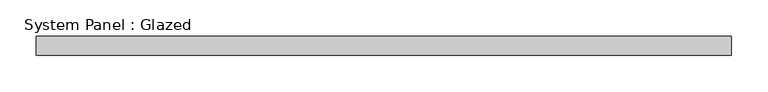
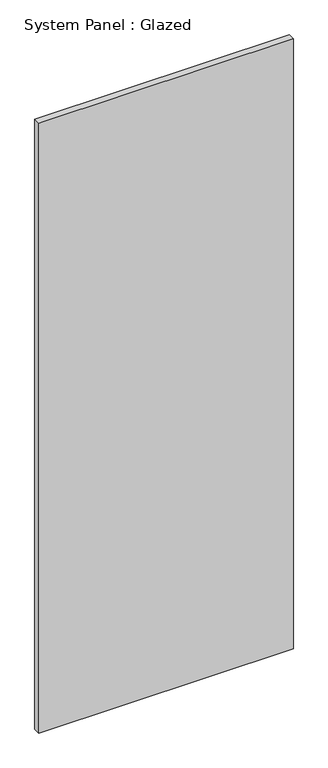
"""IFC4 building model written with IfcOpenShell, lengths in millimetres: plate geometry, System Panel : Glazed."""

from ifc_helpers import new_model, si_unit, origin, origin_with_axes, place, context, project, spatial, polyline, outline, extrude, source, transform, mapped, element, save


def system_panel_glazed_581c84aa(model_context):
    return source(origin(), model_context, "Body", "SweptSolid", [
        extrude(outline(polyline([(476.25, 19.05), (-476.25, 19.05), (-476.25, 44.45), (476.25, 44.45), (476.25, 19.05)])), origin_with_axes(), (0.0, 0.0, 1.0), 2411.6388159),
    ])


if __name__ == "__main__":
    model = new_model("IFC4")
    model_context = context("Model", 3, world=origin())
    ifc_project = project(units=[si_unit("LENGTHUNIT", "METRE", prefix="MILLI")], contexts=[model_context])
    site = spatial("IfcSite", under=ifc_project)
    building = spatial("IfcBuilding", under=site)
    placement = place(None, origin())
    system_panel_glazed_shape = system_panel_glazed_581c84aa(model_context)
    element("IfcPlate", 1, ObjectType="System Panel : Glazed", at=placement, inside=building, context=model_context, shape_type="MappedRepresentation", body=[
        mapped(system_panel_glazed_shape, transform((0.0, 0.0, 0.0), x_axis=(1.0, 0.0, 0.0), y_axis=(0.0, 1.0, 0.0), z_axis=(0.0, 0.0, 1.0))),
    ])
    save(model, "model.ifc")

# Revit data of these elements
# Type "System Panel : Glazed"
#   Construction Type Id = "GSP4R"
#   Analytic Construction = "1/8 in Pilkington single glazing"
#   Visual Light Transmittance = 0.9
#   Solar Heat Gain Coefficient = 0.86
#   Heat Transfer Coefficient (U) = 1.18115 BTU/(h·ft²·°F)
#   Define Thermal Properties by = 1
# Element 1 (IfcPlate, "System Panel : Glazed")
#   Materials on its faces: "Glass"
# Materials
#   "Glass": class "Glass", colour RGB 0 128 192, transparency 0.75, Description = "Soda Lime Glass", Cost = 0
